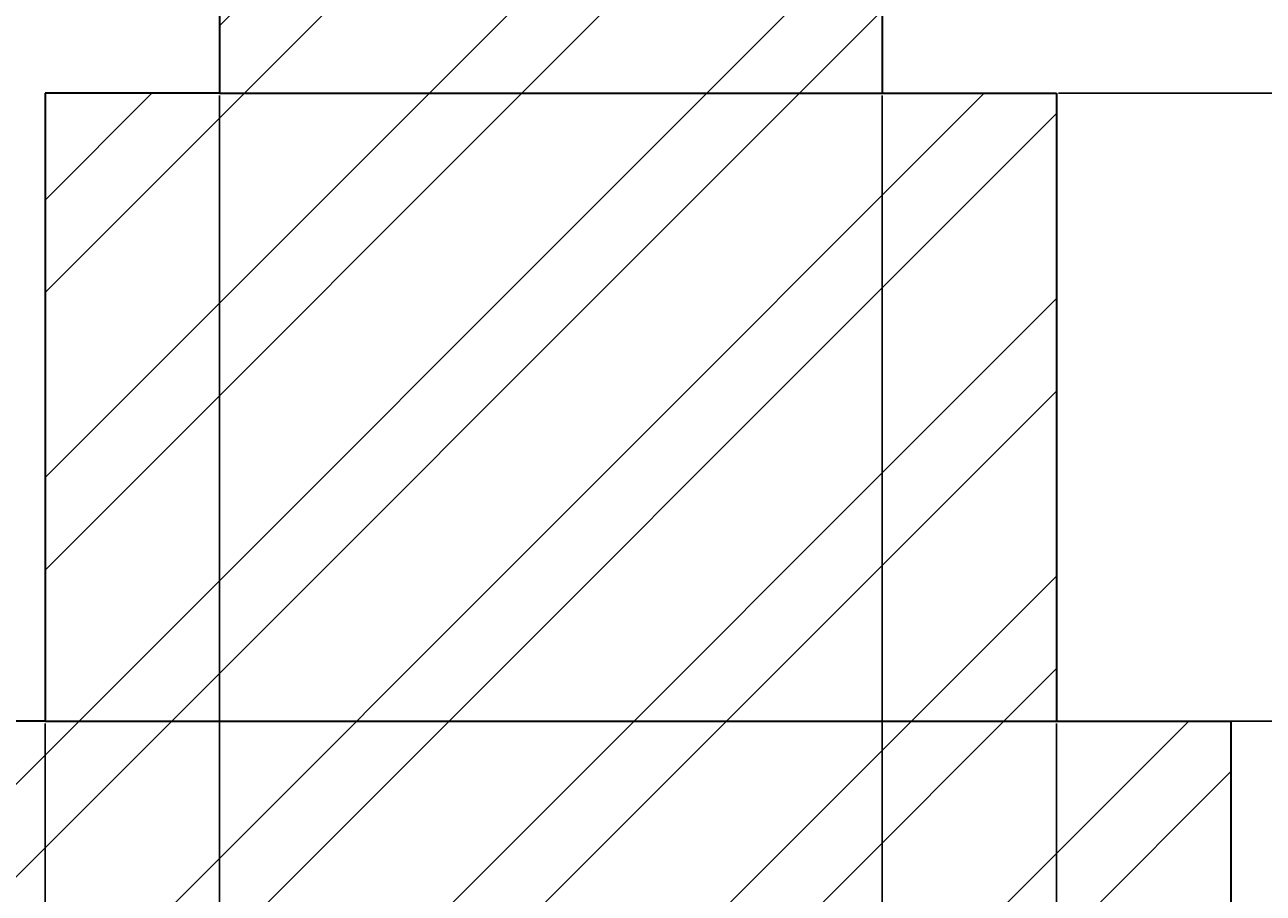
# Model space of a CAD drawing. Units: inches. Extents: x -301 to 715, y -607 to 364.
# Tile 31 of 141: x 124 to 159, y -516 to -492. Entities that reach past the tile are written whole.
import ezdxf

# ---------------------------------------------------------------- set-up
doc = ezdxf.new("R2010")
doc.units = ezdxf.units.IN
doc.header["$MEASUREMENT"] = 0
for name, color, linetype, lineweight in [('A-ANNO-DIMS', 2, 'Continuous', 18), ('A-SECT-PATT', 8, 'Continuous', 13), ('S-FNDN', 2, 'Continuous', 35)]:
    doc.layers.add(name, color=color, linetype=linetype, lineweight=lineweight)
doc.styles.get("Standard").update_dxf_attribs({"font": 'arial.ttf'})
doc.dimstyles.get("Standard").update_dxf_attribs({"dimtxt": 0.18, "dimasz": 0.18, "dimexe": 0.18, "dimexo": 0.0625, "dimgap": 0.09, "dimtad": 0, "dimtih": 1, "dimtoh": 1, "dimdec": 1, "dimzin": 0, "dimdsep": 46, "dimlunit": 4, "dimtxsty": 'Standard', "dimcen": 0.09, "dimclrd": 3, "dimclre": 4, "dimclrt": 6, "dimadec": 0, "dimazin": 0, "dimtfac": 1, "dimtdec": 1, "dimtofl": 0, "dimtmove": 0, "dimatfit": 3, "dimfxl": 1, "dimtfill": 2, "dimtfillclr": 51, "dimtolj": 1, "dimtzin": 0, "dimarcsym": 0})

# ---------------------------------------------------------------- blocks, each defined once
blk = doc.blocks.new('*D78')
at = {"layer": 'A-ANNO-DIMS', "color": 0, "lineweight": -2, "transparency": 16777216}
for p, q in [((158.318, -511.477), (177.276, -511.477)), ((177.096, -516.477), (177.096, -520.877)), ((177.096, -530.477), (177.096, -526.078)), ((158.318, -535.477), (177.276, -535.477))]:
    blk.add_line(p, q, dxfattribs=at)
at = {"layer": 'A-ANNO-DIMS', "color": 0, "transparency": 16777216}
for points in [[(176.262, -516.477), (177.929, -516.477), (177.096, -511.477)], [(176.262, -530.477), (177.929, -530.477), (177.096, -535.477)]]:
    blk.add_solid(points, dxfattribs=at)
at = {"layer": 'Defpoints', "color": 0, "transparency": 16777216}
for p in [(158.255, -511.477), (177.096, -511.477), (158.255, -535.477)]:
    blk.add_point(p, dxfattribs=at)
at = {"layer": 'A-ANNO-DIMS', "color": 0, "transparency": 16777216, "insert": (177.096, -523.477), "char_height": 5, "attachment_point": 5, "bg_fill": 1, "box_fill_scale": 1.25, "bg_fill_color": 51, "bg_fill_transparency": 0}
blk.add_mtext("\\A1;2'", dxfattribs=at)
blk = doc.blocks.new('*D79')
at = {"layer": 'A-ANNO-DIMS', "color": 0, "lineweight": -2, "transparency": 16777216}
for p, q in [((153.318, -493.477), (177.201, -493.477)), ((177.021, -498.477), (177.021, -499.835)), ((177.021, -506.477), (177.021, -505.12)), ((153.318, -511.477), (177.201, -511.477))]:
    blk.add_line(p, q, dxfattribs=at)
at = {"layer": 'A-ANNO-DIMS', "color": 0, "transparency": 16777216}
for points in [[(176.188, -498.477), (177.854, -498.477), (177.021, -493.477)], [(176.188, -506.477), (177.854, -506.477), (177.021, -511.477)]]:
    blk.add_solid(points, dxfattribs=at)
at = {"layer": 'Defpoints', "color": 0, "transparency": 16777216}
for p in [(153.255, -493.477), (177.021, -493.477), (153.255, -511.477)]:
    blk.add_point(p, dxfattribs=at)
at = {"layer": 'A-ANNO-DIMS', "color": 0, "transparency": 16777216, "insert": (177.021, -502.477), "char_height": 5, "attachment_point": 5, "bg_fill": 1, "box_fill_scale": 1.25, "bg_fill_color": 51, "bg_fill_transparency": 0}
blk.add_mtext('\\A1;1\'-6"', dxfattribs=at)
blk = doc.blocks.new('*D80')
at = {"layer": 'A-ANNO-DIMS', "color": 0, "lineweight": -2, "transparency": 16777216}
for p, q in [((176.814, -481.477), (176.814, -476.477)), ((176.814, -476.477), (181.814, -476.477)), ((153.318, -481.477), (176.994, -481.477)), ((176.814, -488.477), (176.814, -486.477)), ((153.318, -493.477), (176.994, -493.477))]:
    blk.add_line(p, q, dxfattribs=at)
at = {"layer": 'A-ANNO-DIMS', "color": 0, "transparency": 16777216}
for points in [[(175.981, -486.477), (177.648, -486.477), (176.814, -481.477)], [(175.981, -488.477), (177.648, -488.477), (176.814, -493.477)]]:
    blk.add_solid(points, dxfattribs=at)
at = {"layer": 'Defpoints', "color": 0, "transparency": 16777216}
for p in [(153.255, -481.477), (176.814, -481.477), (153.255, -493.477)]:
    blk.add_point(p, dxfattribs=at)
at = {"layer": 'A-ANNO-DIMS', "color": 0, "transparency": 16777216, "insert": (183.969, -476.477), "char_height": 5, "attachment_point": 5, "bg_fill": 1, "box_fill_scale": 1.25, "bg_fill_color": 51, "bg_fill_transparency": 0}
blk.add_mtext("\\A1;1'", dxfattribs=at)
blk = doc.blocks.new('*D176')
at = {"layer": 'A-ANNO-DIMS', "color": 4, "lineweight": -2, "transparency": 16777216}
for p, q in [((148.28, -324.477), (215.605, -324.477)), ((-15.22, -540.477), (215.605, -540.477))]:
    blk.add_line(p, q, dxfattribs=at)
at = {"layer": 'A-ANNO-DIMS', "color": 3, "lineweight": -2, "transparency": 16777216}
for p, q in [((215.425, -324.657), (215.425, -432.296)), ((215.425, -540.297), (215.425, -432.659))]:
    blk.add_line(p, q, dxfattribs=at)
at = {"layer": 'A-ANNO-DIMS', "color": 3, "transparency": 16777216}
for points in [[(215.395, -324.657), (215.455, -324.657), (215.425, -324.477)], [(215.395, -540.297), (215.455, -540.297), (215.425, -540.477)]]:
    blk.add_solid(points, dxfattribs=at)
at = {"layer": 'Defpoints', "color": 0, "transparency": 16777216}
for p in [(148.218, -324.477), (-15.282, -540.477), (215.425, -540.477)]:
    blk.add_point(p, dxfattribs=at)
at = {"layer": 'A-ANNO-DIMS', "color": 6, "transparency": 16777216, "insert": (215.425, -432.477), "char_height": 0.18, "attachment_point": 5, "bg_fill": 1, "box_fill_scale": 1.25, "bg_fill_color": 51, "bg_fill_transparency": 0}
blk.add_mtext('\\A1;18\'-0"', dxfattribs=at)
blk = doc.blocks.new('*D184')
at = {"layer": 'A-ANNO-DIMS', "color": 4, "lineweight": -2, "transparency": 16777216}
for p, q in [((124.255, -511.54), (124.255, -573.809)), ((153.255, -511.54), (153.255, -573.809))]:
    blk.add_line(p, q, dxfattribs=at)
at = {"layer": 'A-ANNO-DIMS', "color": 3, "lineweight": -2, "transparency": 16777216}
for p, q in [((124.435, -573.629), (138.424, -573.629)), ((153.075, -573.629), (139.086, -573.629))]:
    blk.add_line(p, q, dxfattribs=at)
at = {"layer": 'A-ANNO-DIMS', "color": 3, "transparency": 16777216}
for points in [[(124.435, -573.599), (124.435, -573.659), (124.255, -573.629)], [(153.075, -573.599), (153.075, -573.659), (153.255, -573.629)]]:
    blk.add_solid(points, dxfattribs=at)
at = {"layer": 'Defpoints', "color": 0, "transparency": 16777216}
for p in [(124.255, -511.477), (153.255, -511.477), (153.255, -573.629)]:
    blk.add_point(p, dxfattribs=at)
at = {"layer": 'A-ANNO-DIMS', "color": 6, "transparency": 16777216, "insert": (138.755, -573.629), "char_height": 0.18, "attachment_point": 5, "bg_fill": 1, "box_fill_scale": 1.25, "bg_fill_color": 51, "bg_fill_transparency": 0}
blk.add_mtext('\\A1;2\'-5"', dxfattribs=at)
blk = doc.blocks.new('*D185')
at = {"layer": 'A-ANNO-DIMS', "color": 4, "lineweight": -2, "transparency": 16777216}
for p, q in [((129.255, -493.54), (129.255, -573.809)), ((148.255, -493.54), (148.255, -573.809))]:
    blk.add_line(p, q, dxfattribs=at)
at = {"layer": 'A-ANNO-DIMS', "color": 3, "lineweight": -2, "transparency": 16777216}
for p, q in [((129.435, -573.629), (138.434, -573.629)), ((148.075, -573.629), (139.076, -573.629))]:
    blk.add_line(p, q, dxfattribs=at)
at = {"layer": 'A-ANNO-DIMS', "color": 3, "transparency": 16777216}
for points in [[(129.435, -573.599), (129.435, -573.659), (129.255, -573.629)], [(148.075, -573.599), (148.075, -573.659), (148.255, -573.629)]]:
    blk.add_solid(points, dxfattribs=at)
at = {"layer": 'Defpoints', "color": 0, "transparency": 16777216}
for p in [(129.255, -493.477), (148.255, -493.477), (148.255, -573.629)]:
    blk.add_point(p, dxfattribs=at)
at = {"layer": 'A-ANNO-DIMS', "color": 6, "transparency": 16777216, "insert": (138.755, -573.629), "char_height": 0.18, "attachment_point": 5, "bg_fill": 1, "box_fill_scale": 1.25, "bg_fill_color": 51, "bg_fill_transparency": 0}
blk.add_mtext('\\A1;1\'-7"', dxfattribs=at)
blk = doc.blocks.new('*D190')
at = {"layer": 'A-ANNO-DIMS', "color": 4, "lineweight": -2, "transparency": 16777216}
for p, q in [((129.193, -481.477), (-266.112, -481.477)), ((124.193, -511.477), (-266.112, -511.477))]:
    blk.add_line(p, q, dxfattribs=at)
at = {"layer": 'A-ANNO-DIMS', "color": 3, "lineweight": -2, "transparency": 16777216}
for p, q in [((-265.932, -481.657), (-265.932, -496.296)), ((-265.932, -511.297), (-265.932, -496.659))]:
    blk.add_line(p, q, dxfattribs=at)
at = {"layer": 'A-ANNO-DIMS', "color": 3, "transparency": 16777216}
for points in [[(-265.962, -481.657), (-265.902, -481.657), (-265.932, -481.477)], [(-265.962, -511.297), (-265.902, -511.297), (-265.932, -511.477)]]:
    blk.add_solid(points, dxfattribs=at)
at = {"layer": 'Defpoints', "color": 0, "transparency": 16777216}
for p in [(129.255, -481.477), (-265.932, -511.477), (124.255, -511.477)]:
    blk.add_point(p, dxfattribs=at)
at = {"layer": 'A-ANNO-DIMS', "color": 6, "transparency": 16777216, "insert": (-265.932, -496.477), "char_height": 0.18, "attachment_point": 5, "bg_fill": 1, "box_fill_scale": 1.25, "bg_fill_color": 51, "bg_fill_transparency": 0}
blk.add_mtext('\\A1;2\'-6"', dxfattribs=at)
blk = doc.blocks.new('*D191')
at = {"layer": 'A-ANNO-DIMS', "color": 4, "lineweight": -2, "transparency": 16777216}
for p, q in [((129.193, -481.477), (-266.112, -481.477)), ((114.193, -540.477), (-266.112, -540.477))]:
    blk.add_line(p, q, dxfattribs=at)
at = {"layer": 'A-ANNO-DIMS', "color": 3, "lineweight": -2, "transparency": 16777216}
for p, q in [((-265.932, -481.657), (-265.932, -510.797)), ((-265.932, -540.297), (-265.932, -511.158))]:
    blk.add_line(p, q, dxfattribs=at)
at = {"layer": 'A-ANNO-DIMS', "color": 3, "transparency": 16777216}
for points in [[(-265.962, -481.657), (-265.902, -481.657), (-265.932, -481.477)], [(-265.962, -540.297), (-265.902, -540.297), (-265.932, -540.477)]]:
    blk.add_solid(points, dxfattribs=at)
at = {"layer": 'Defpoints', "color": 0, "transparency": 16777216}
for p in [(129.255, -481.477), (-265.932, -540.477), (114.255, -540.477)]:
    blk.add_point(p, dxfattribs=at)
at = {"layer": 'A-ANNO-DIMS', "color": 6, "transparency": 16777216, "insert": (-265.932, -510.977), "char_height": 0.18, "attachment_point": 5, "bg_fill": 1, "box_fill_scale": 1.25, "bg_fill_color": 51, "bg_fill_transparency": 0}
blk.add_mtext('\\A1;4\'-11"', dxfattribs=at)

msp = doc.modelspace()

# ---------------------------------------------------------------- hatches: boundary and pattern name
at = {"layer": 'A-SECT-PATT'}
h = msp.add_hatch(dxfattribs=at)
h.set_pattern_fill('ANSI32', color=256, scale=15)
h.set_pattern_definition([(45, (10.321, 33.8764), (-3.977476, 3.977476), []), (45, (12.973, 33.8764), (-3.977476, 3.977476), [])])
h.paths.add_polyline_path([(-185.282, -324.477), (-199.282, -324.477), (-199.282, -329.477), (-194.282, -329.477), (-194.282, -353.477), (-185.282, -353.477)])
h.paths.add_polyline_path([(-185.282, -361.477), (-193.904, -361.477), (-193.982, -377.537), (-185.282, -377.537)])
h.paths.add_polyline_path([(143.218, -329.477), (148.218, -329.477), (148.218, -324.477), (134.255, -324.477), (134.255, -353.477), (143.218, -353.477)])
h.paths.add_polyline_path([(143.218, -361.477), (134.255, -361.477), (134.255, -377.477), (143.218, -377.477)])
h.paths.add_polyline_path([(-185.282, -439.477), (-194.282, -439.477), (-194.282, -463.477), (-185.282, -463.477)])
h.paths.add_polyline_path([(-185.282, -471.477), (-194.282, -471.477), (-194.282, -481.477), (-185.282, -481.477)])
h.paths.add_polyline_path([(-185.282, -463.477), (-194.282, -463.477), (-194.282, -466.477), (-185.282, -466.477)])
h.paths.add_polyline_path([(-185.282, -466.477), (-194.282, -466.477), (-194.282, -471.477), (-185.282, -471.477)])
h.paths.add_polyline_path([(-180.282, -481.477), (-185.282, -481.477), (-194.282, -481.477), (-199.282, -481.477), (-199.282, -493.477), (-180.282, -493.477)])
h.paths.add_polyline_path([(-175.282, -493.477), (-180.282, -493.477), (-199.282, -493.477), (-204.282, -493.477), (-204.282, -511.477), (-175.282, -511.477)])
h.paths.add_polyline_path([(-170.282, -511.477), (-175.282, -511.477), (-204.282, -511.477), (-209.282, -511.477), (-209.282, -535.477), (-170.282, -535.477)])
h.paths.add_polyline_path([(-35.282, -463.477), (-41.282, -463.477), (-41.282, -466.477), (-35.282, -466.477)])
h.paths.add_polyline_path([(-35.282, -466.477), (-41.282, -466.477), (-41.282, -471.477), (-35.282, -471.477)])
h.paths.add_polyline_path([(-35.282, -471.477), (-41.282, -471.477), (-41.282, -481.477), (-35.282, -481.477)])
h.paths.add_polyline_path([(-30.282, -481.477), (-46.282, -481.477), (-46.282, -493.477), (-30.282, -493.477)])
h.paths.add_polyline_path([(-25.282, -493.477), (-30.282, -493.477), (-46.282, -493.477), (-51.282, -493.477), (-51.282, -511.477), (-25.282, -511.477)])
h.paths.add_polyline_path([(-20.282, -511.477), (-25.282, -511.477), (-51.282, -511.477), (-56.282, -511.477), (-56.282, -535.477), (-20.282, -535.477)])
h.paths.add_polyline_path([(143.218, -463.477), (134.255, -463.477), (134.255, -466.477), (143.218, -466.477)])
h.paths.add_polyline_path([(143.218, -466.477), (134.255, -466.477), (134.255, -471.477), (143.218, -471.477)])
h.paths.add_polyline_path([(143.218, -471.477), (134.255, -471.477), (134.255, -481.477), (143.218, -481.477)])
h.paths.add_polyline_path([(148.255, -481.477), (143.255, -481.477), (134.255, -481.477), (129.255, -481.477), (129.255, -493.477), (148.255, -493.477)])
h.paths.add_polyline_path([(153.255, -493.477), (148.255, -493.477), (129.255, -493.477), (124.255, -493.477), (124.255, -511.477), (153.255, -511.477)])
h.paths.add_polyline_path([(158.255, -511.477), (153.255, -511.477), (124.255, -511.477), (119.255, -511.477), (119.255, -535.477), (158.255, -535.477)])

# ---------------------------------------------------------------- linework, layer by layer
at = {"layer": 'S-FNDN'}
for p, q in [((129.255, -481.477), (129.255, -493.477)), ((148.255, -481.477), (148.255, -493.477)), ((129.255, -493.477), (124.255, -493.477)), ((124.255, -493.477), (124.255, -511.477)), ((129.255, -493.477), (148.255, -493.477)), ((148.255, -493.477), (153.255, -493.477)), ((153.255, -493.477), (153.255, -511.477)), ((124.255, -511.477), (119.255, -511.477)), ((124.255, -511.477), (153.255, -511.477)), ((153.255, -511.477), (158.255, -511.477)), ((158.255, -511.477), (158.255, -535.477))]:
    msp.add_line(p, q, dxfattribs=at)

# ---------------------------------------------------------------- dimensions: what is measured, and where the dimension line sits
at = {"layer": 'A-ANNO-DIMS'}
for base, p1, p2, override, picture, middle in [((215.425, -540.477), (148.218, -324.477), (-15.282, -540.477), {"dimdec": 1, "dimlfac": 1, "dimrnd": 0, "dimzin": 1, "dimdsep": 46, "dimlunit": 4, "dimfrac": 2}, '*D176', (215.425, -432.477)), ((176.814, -481.477), (153.255, -493.477), (153.255, -481.477), {"dimtxt": 5, "dimasz": 5, "dimclrd": 0, "dimclre": 0, "dimclrt": 0}, '*D80', (183.969, -476.477)), ((-265.932, -540.477), (129.255, -481.477), (114.255, -540.477), {"dimdec": 1, "dimlfac": 1, "dimrnd": 0, "dimzin": 1, "dimdsep": 46, "dimlunit": 4, "dimfrac": 2}, '*D191', (-265.932, -510.977)), ((-265.932, -511.477), (129.255, -481.477), (124.255, -511.477), {"dimdec": 1, "dimlfac": 1, "dimrnd": 0, "dimzin": 1, "dimdsep": 46, "dimlunit": 4, "dimfrac": 2}, '*D190', (-265.932, -496.477)), ((177.021, -493.477), (153.255, -511.477), (153.255, -493.477), {"dimtxt": 5, "dimasz": 5, "dimclrd": 0, "dimclre": 0, "dimclrt": 0}, '*D79', (177.021, -502.477)), ((177.096, -511.477), (158.255, -535.477), (158.255, -511.477), {"dimtxt": 5, "dimasz": 5, "dimclrd": 0, "dimclre": 0, "dimclrt": 0}, '*D78', (177.096, -523.477))]:
    dim = msp.add_linear_dim(base=base, p1=p1, p2=p2, angle=90, dimstyle='Standard', override=override, dxfattribs=at)
    dim.commit()
    dim.dimension.update_dxf_attribs({"geometry": picture, "text_midpoint": middle})
for base, p1, p2, picture in [((148.255, -573.629), (129.255, -493.477), (148.255, -493.477), '*D185'), ((153.255, -573.629), (124.255, -511.477), (153.255, -511.477), '*D184')]:
    dim = msp.add_linear_dim(base=base, p1=p1, p2=p2, dimstyle='Standard', override={"dimdec": 1, "dimlfac": 1, "dimrnd": 0, "dimzin": 1, "dimdsep": 46, "dimlunit": 4, "dimfrac": 2}, dxfattribs=at)
    dim.commit()
    dim.dimension.update_dxf_attribs({"geometry": picture, "text_midpoint": (138.755, -573.629)})

doc.saveas('drawing.dxf')
